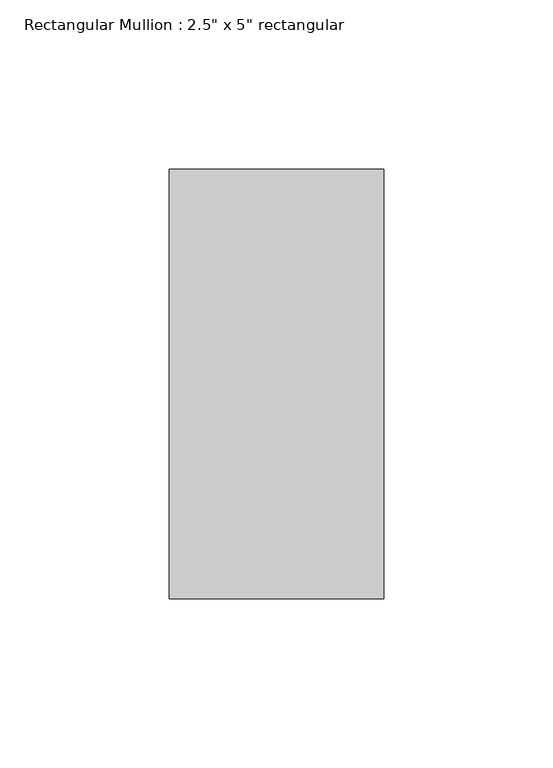
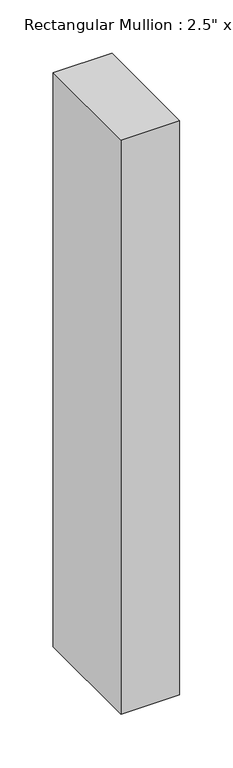
"""IFC4 building model written with IfcOpenShell, lengths in millimetres: member geometry."""

from ifc_helpers import new_model, si_unit, frame, origin, place, context, project, spatial, polyline, outline, extrude, source, transform, mapped, element, save


def member_43a8b99b(model_context):
    return source(origin(), model_context, "Body", "SweptSolid", [
        extrude(outline(polyline([(0.0, 63.5), (0.0, -63.5), (-63.5, -63.5), (-63.5, 63.5), (0.0, 63.5)])), frame((0.0, 0.0, -656.4208479), z_axis=(0.0, 0.0, 1.0), x_axis=(1.0, 0.0, 0.0)), (0.0, 0.0, 1.0), 656.4208479),
    ])


if __name__ == "__main__":
    model = new_model("IFC4")
    model_context = context("Model", 3, world=origin())
    ifc_project = project(units=[si_unit("LENGTHUNIT", "METRE", prefix="MILLI")], contexts=[model_context])
    site = spatial("IfcSite", under=ifc_project)
    building = spatial("IfcBuilding", under=site)
    placement = place(None, origin())
    member_shape = member_43a8b99b(model_context)
    element("IfcMember", 1, ObjectType="Rectangular Mullion : 2.5\" x 5\" rectangular", at=placement, inside=building, context=model_context, shape_type="MappedRepresentation", body=[
        mapped(member_shape, transform((0.0, 0.0, 0.0), x_axis=(1.0, 0.0, 0.0), y_axis=(0.0, 1.0, 0.0), z_axis=(0.0, 0.0, 1.0))),
    ])
    save(model, "model.ifc")

# Revit data of these elements
# Type "Rectangular Mullion : 2.5\" x 5\" rectangular"
#   built-in parameter 1007304 = 0.416667 (stored number, unit not read)
#   built-in parameter 1007301 = 0.104167 (stored number, unit not read)
#   built-in parameter 1007300 = 0.104167 (stored number, unit not read)
# Element 1 (IfcMember, "Rectangular Mullion : 2.5\" x 5\" rectangular")
#   Materials on its faces: "Aluminum"
# Materials
#   "Aluminum": class "Metal", colour RGB 247 247 247, transparency 0, Description = "Aluminum 6061", Cost = 0
